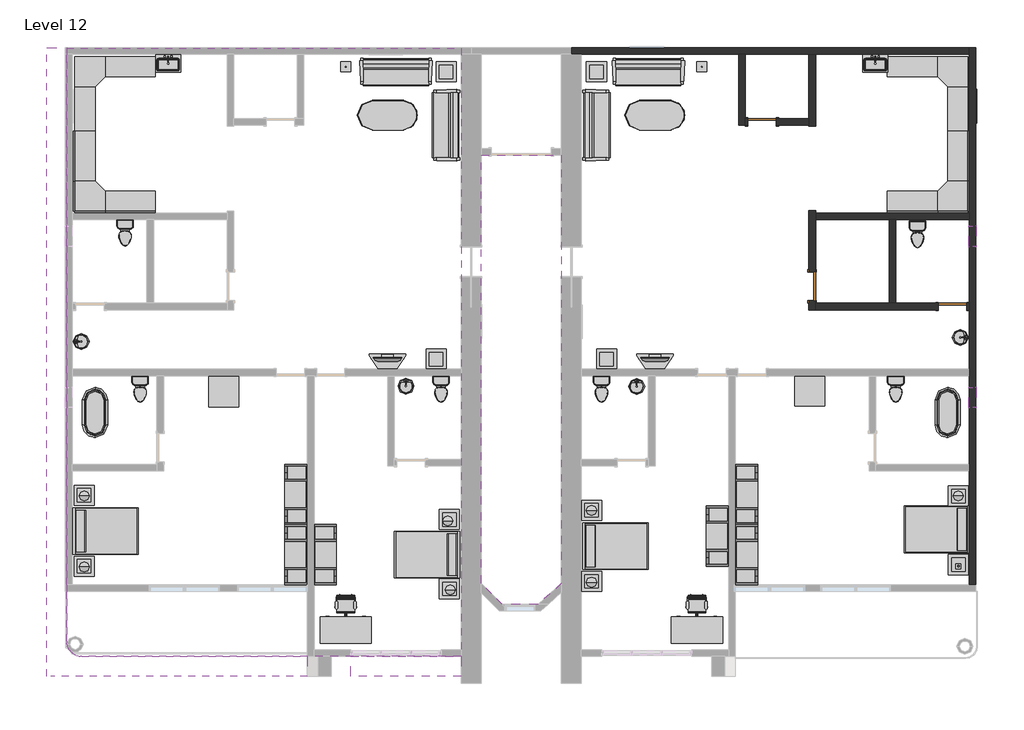
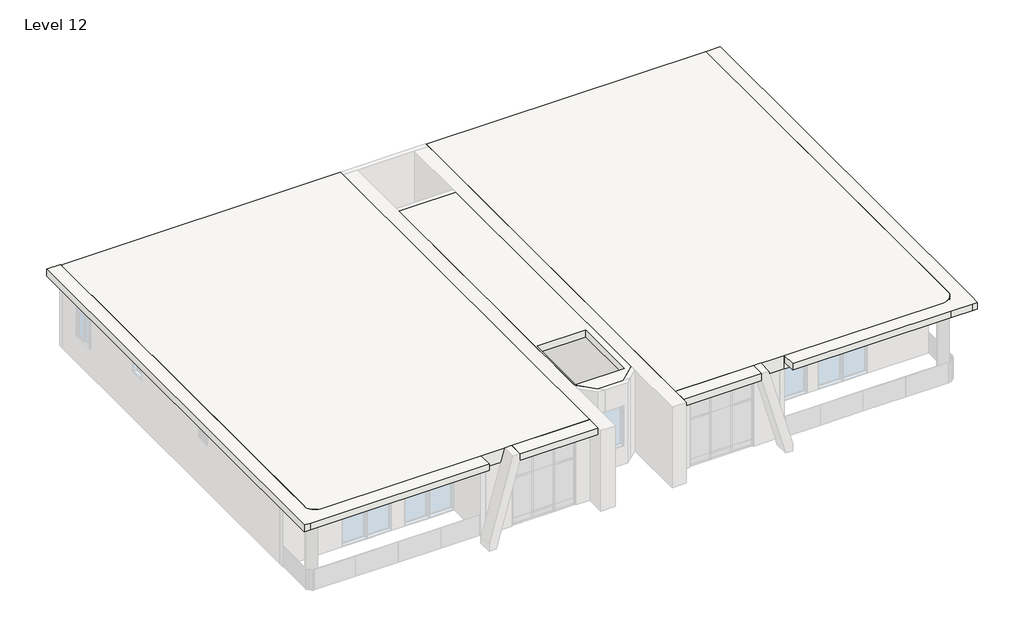
# One storey, part 3 of 3: 42 furniture elements, 14 flow terminals, 10 light fixtures, 9 walls, 4 slabs, 3 doors, 3 windows.
# Revit data of these elements (continued)
# Elements 26, 27 (IfcFurniture, "Desk : 60\" x 30\"")
#   Phase Created = New Construction
#   Materials on its faces: "Steel, Chrome Plated", "Laminate, Ivory, Matte", "Cherry"
# Elements 28, 29, 30, 31, 32, 33 (IfcFurniture, "Entertainment Center : 72\" x 72\" x 24\"")
#   Phase Created = New Construction
#   Materials on its faces: "Steel, Chrome Plated", "Glass - Clear, Grey"
# Elements 34, 35, 36, 37 (IfcFurniture, "Sofa-Pensi : 84\"")
#   Phase Created = New Construction
#   Materials on its faces: "Cherry", "Linen, Beige", "Steel, Chrome Plated"
# Elements 38, 39 (IfcFurniture, "TV - Flat Screen : 32\"")
#   Stand = yes
#   Phase Created = New Construction
#   Materials on its faces: "TV - Black", "TV - Glass", "TV - Screen"
# Elements 40, 41 (IfcFurniture, "TV Stand : TV Stand")
#   Phase Created = New Construction
#   Materials on its faces: "Melamine - Gray", "Glass - Shelves"
# Elements 42, 43, 44, 45, 46, 47, 48, 49, 50, 51, 52, 53 (IfcFurniture, "Table-Coffee : 24\" x 24\" x 24\"")
#   Phase Created = New Construction
#   Materials on its faces: "Glass - Clear, Grey"
# Elements 54, 55 (IfcFurniture, "Table-Dining Oval : 36\" x 72\"")
#   Phase Created = New Construction
#   Materials on its faces: "Steel, Chrome Plated", "Glass - Clear, Grey"
# Elements 56, 57 (IfcFurniture, "Table-Rectangular : 36\" x 36\"")
#   Phase Created = New Construction
#   Materials on its faces: "Birch"
# Elements 58, 59 (IfcFurniture, "Work Station Cubicle : 96\" x 96\"")
#   Phase Created = New Construction
#   Materials on its faces: "Textile - Light Gray", "Laminate, Ivory, Matte"
# Element 60 (IfcLightFixture, "100W - 120V")
#   Mark = "134"
#   Phase Created = New Construction
#   Materials on its faces: "Steel, Chrome Plated", "Glass, Frosted"
# Element 61 (IfcLightFixture, "100W - 120V")
#   Mark = "135"
#   Phase Created = New Construction
#   Materials on its faces: "Steel, Chrome Plated", "Glass, Frosted"
# Element 62 (IfcLightFixture, "Table Lamp - Hemispheric : 60W - 120V")
#   Mark = "136"
#   Phase Created = New Construction
#   Materials on its faces: "Steel, Chrome Plated", "Glass, Frosted", "Birch"
# Element 63 (IfcLightFixture, "Table Lamp - Hemispheric : 60W - 120V")
#   Mark = "137"
#   Phase Created = New Construction
#   Materials on its faces: "Steel, Chrome Plated", "Glass, Frosted", "Birch"
# Element 64 (IfcLightFixture, "Table Lamp - Hemispheric : 60W - 120V")
#   Mark = "138"
#   Phase Created = New Construction
#   Materials on its faces: "Steel, Chrome Plated", "Glass, Frosted", "Birch"
# Element 65 (IfcLightFixture, "Table Lamp - Hemispheric : 60W - 120V")
#   Mark = "139"
#   Phase Created = New Construction
#   Materials on its faces: "Steel, Chrome Plated", "Glass, Frosted", "Birch"
# Element 66 (IfcLightFixture, "Table Lamp - Hemispheric : 60W - 120V")
#   Mark = "140"
#   Phase Created = New Construction
#   Materials on its faces: "Steel, Chrome Plated", "Glass, Frosted", "Birch"
# Element 67 (IfcLightFixture, "Table Lamp - Hemispheric : 60W - 120V")
#   Mark = "141"
#   Phase Created = New Construction
#   Materials on its faces: "Steel, Chrome Plated", "Glass, Frosted", "Birch"
# Element 68 (IfcLightFixture, "Table Lamp - Hemispheric : 60W - 120V")
#   Mark = "142"
#   Phase Created = New Construction
#   Materials on its faces: "Steel, Chrome Plated", "Glass, Frosted", "Birch"
# Element 69 (IfcLightFixture, "Table Lamp - Hemispheric : 60W - 120V")
#   Mark = "143"
#   Phase Created = New Construction
#   Materials on its faces: "Steel, Chrome Plated", "Glass, Frosted", "Birch"
# Element 70 (IfcSlab, "Generic - 12\" cream")
#   Height Offset From Level = 12' - 0"
#   Phase Created = New Construction
#   Materials on its faces: "Parking Stripe"
# Element 71 (IfcSlab, "Generic - 12\" white")
#   built-in parameter 1001955 = 3.14159 (stored number, unit not read)
#   Height Offset From Level = 12' - 0"
#   Phase Created = New Construction
#   Materials on its faces: "Door - Frame"
# Elements 72, 73 (IfcSlab, "Generic - 12\" white")
#   Height Offset From Level = 12' - 0"
#   Phase Created = New Construction
#   Materials on its faces: "Door - Frame"
# Elements 74, 75, 76, 77, 78, 79, 80, 81 (IfcWall, "Generic - 8\" cream")
#   Top Offset = 0' - 0"
#   Base Offset = 0' - 0"
#   Unconnected Height = 10' - 0"
#   wall height = 10' - 0"
#   Phase Created = New Construction
#   Base Constraint = Level 12
#   Materials on its faces: "Parking Stripe"
# Element 82 (IfcWall, "Generic - 8\" white")
#   Top Offset = 0' - 0"
#   Base Offset = 0' - 0"
#   Unconnected Height = 10' - 0"
#   wall height = 10' - 0"
#   Phase Created = New Construction
#   Base Constraint = Level 12
#   Materials on its faces: "Door - Frame", "Parking Stripe"
# Element 83 (IfcWindow, "Louvers with Trim : 24\" x 24\"")
#   Mark = "262"
#   Phase Created = New Construction
#   Materials on its faces: "Glass", "Iron, Ductile"
# Element 84 (IfcWindow, "Louvers with Trim : 24\" x 24\"")
#   Mark = "263"
#   Phase Created = New Construction
#   Materials on its faces: "Glass", "Iron, Ductile"
# Element 85 (IfcWindow, "Slider with Trim : 36\" x 48\"")
#   Mark = "259"
#   Phase Created = New Construction
#   Materials on its faces: "Iron, Ductile", "Glass"
# Materials
#   "Wood - Birch - Solid Stained Light Low Gloss": class "Wood", colour RGB 210 159 95, transparency 0, Cost = 0
#   "Paint - Sienna": colour RGB 118 70 51, transparency 0, Cost = 0
#   "Steel, Polished": class "Metal", colour RGB 57 57 57, transparency 0, Description = "Polished steel", Cost = 0
#   "Porcelain, Linen": class "Ceramic", colour RGB 249 239 230, transparency 0, Description = "Porcelain, linen", Cost = 0
#   "Laminate, Linen, Matte": class "Plastic", colour RGB 249 239 230, transparency 0, Description = "Plastic Laminate - Linen, Matte", Cost = 0
#   "Porcelain, Ivory": class "Ceramic", colour RGB 247 247 239, transparency 0, Description = "Porcelain, ivory", Cost = 0
#   "Laminate, Ivory, Matte": class "Plastic", colour RGB 247 247 239, transparency 0, Description = "Plastic Laminate - Ivory, Matte", Cost = 0
#   "Birch": class "Wood", colour RGB 224 178 126, transparency 0, Description = "Betula Alleghaniensis", Cost = 0
#   "Linen, White": class "Textile", colour RGB 247 247 239, transparency 0, Description = "Linen, white", Cost = 0
#   "Plastic, Opaque Black": class "Plastic", colour RGB 0 0 0, transparency 0.7, Description = "Plastic, generic, opaque black", Cost = 0
#   "Textile - Slate Blue": class "Fabric", colour RGB 98 102 118, transparency 0
#   "Steel, Chrome Plated": class "Metal", colour RGB 17 17 17, transparency 0, Description = "Chromiuim plated steel", Cost = 0
#   "Cherry": class "Wood", colour RGB 226 177 128, transparency 0, Description = "Prunus Serotina", Cost = 0
#   "Linen, Beige": class "Textile", colour RGB 249 239 230, transparency 0, Description = "Linen, beige", Cost = 0
#   "Melamine - Gray": class "Wood", colour RGB 49 49 49, transparency 0
#   "Glass - Clear, Grey": class "Glass", colour RGB 252 255 255, transparency 0.64
#   "Textile - Light Gray": class "Fabric", colour RGB 204 204 204, transparency 0
#   "Glass, Frosted": class "Glass", colour RGB 250 244 225, transparency 0.55, Description = "physical material", Cost = 0
#   "Parking Stripe": class "Paint", colour RGB 250 250 91, transparency 0, Cost = 0
#   "Door - Frame": colour RGB 118 70 51, transparency 0, Cost = 0
#   "Iron, Ductile": class "Metal", colour RGB 0 0 0, transparency 0, Description = "Ductile cast iron", Cost = 0
#   "Glass": class "Glass", colour RGB 0 128 192, transparency 0.75, Description = "Soda Lime Glass", Cost = 0
#   "TV - Black": colour RGB 49 49 49, transparency 0
#   "TV - Glass": colour RGB 157 157 157, transparency 0.9
#   "TV - Screen": colour RGB 0 0 0, transparency 0
#   "Glass - Shelves": class "Glass", colour RGB 167 167 167, transparency 0.9
